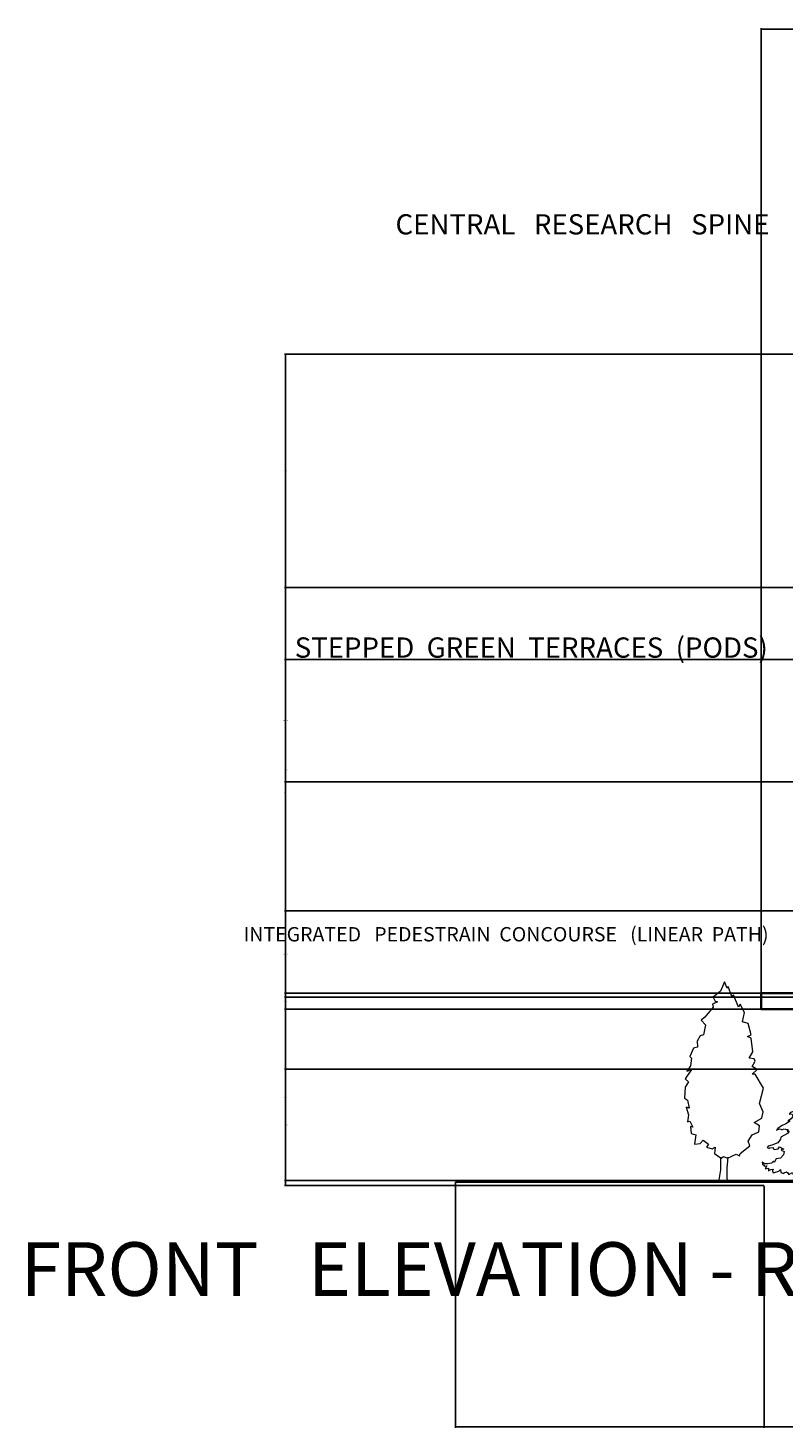
# Model space of a CAD drawing. Units: inches. Extents: x -160 to 434, y -145 to 103.
# Tile 1 of 7: x -160 to -26, y -145 to 103. Entities that reach past the tile are written whole.
import ezdxf

# ---------------------------------------------------------------- set-up
doc = ezdxf.new("R2010")
doc.units = ezdxf.units.IN
doc.header["$MEASUREMENT"] = 0
for name, color, linetype, lineweight in [('A-ANNO-DIMS', 2, 'Continuous', 18), ('A-ANNO-TEXT', 3, 'Continuous', 18), ('A-ELEV', 7, 'Continuous', 35), ('L-PLNT', 3, 'Continuous', 13)]:
    doc.layers.add(name, color=color, linetype=linetype, lineweight=lineweight)
doc.styles.get("Standard").update_dxf_attribs({"font": 'arial.ttf'})
doc.dimstyles.get("Standard").update_dxf_attribs({"dimtxt": 0.18, "dimasz": 0.18, "dimexe": 0.18, "dimexo": 0.0625, "dimgap": 0.09, "dimtad": 0, "dimtih": 1, "dimtoh": 1, "dimdec": 4, "dimzin": 0, "dimdsep": 46, "dimtxsty": 'Standard', "dimcen": 0.09, "dimadec": 0, "dimazin": 0, "dimtfac": 1, "dimtdec": 4, "dimtofl": 0, "dimtmove": 0, "dimatfit": 3, "dimfxl": 1, "dimtolj": 1, "dimtzin": 0, "dimarcsym": 0})

# ---------------------------------------------------------------- blocks, each defined once
blk = doc.blocks.new('*U2')
blk.add_lwpolyline([(-2.754, 191.699), (-6.78, 182.851), (-13.682, 176.953), (-11.956, 173.266), (-9.656, 172.529), (-14.257, 170.317), (-13.682, 167.368), (-21.733, 157.783), (-25.184, 154.834), (-21.158, 150.41), (-21.733, 147.461), (-22.884, 140.825), (-26.334, 140.087), (-29.21, 134.926), (-28.635, 129.028), (-32.661, 128.291), (-36.111, 120.18), (-34.386, 118.706), (-35.536, 111.333), (-38.987, 106.171), (-34.386, 107.646), (-40.712, 98.798), (-37.261, 95.849), (-40.712, 90.688), (-41.287, 80.366), (-38.412, 78.154), (-36.686, 70.781), (-39.562, 71.518), (-37.261, 64.145), (-38.412, 57.509), (-36.111, 58.247), (-33.236, 52.348), (-35.536, 53.086), (-34.961, 46.45), (-30.36, 44.975), (-31.51, 36.128), (-26.334, 36.865), (-23.459, 39.814), (-18.283, 36.128), (-20.008, 33.178), (-14.832, 31.704), (-11.956, 33.178), (-12.531, 27.28), (-6.205, 22.856), (-3.905, 24.331), (0.121, 22.856), (8.173, 26.543), (11.624, 25.068), (12.199, 27.28), (21.4, 34.653), (19.675, 39.077), (23.701, 44.975), (30.027, 47.924), (30.602, 53.823), (25.426, 56.772), (32.903, 61.196), (34.053, 67.094), (30.602, 75.205), (34.628, 89.951), (26.576, 103.222), (23.701, 103.222), (28.302, 107.646), (23.701, 110.595), (26.576, 115.756), (25.426, 117.968), (20.825, 118.706), (24.276, 124.604), (22.551, 137.876), (19.1, 139.35), (22.551, 140.825), (19.675, 151.884), (14.499, 153.359), (16.224, 162.207), (12.199, 170.317), (10.473, 167.368), (5.872, 179.165), (4.147, 177.69), (0.696, 187.275), (-0.454, 185.8)], close=True)
for points in [[(-6.813, 23.669), (-6.813, 11.669), (-8.627, 0)], [(0.387, 23.669), (-0.576, 13.271), (-0.576, 3.686), (0, 0)]]:
    blk.add_lwpolyline(points)
blk = doc.blocks.new('*U7')
for p, q in [((-9.75, 0), (-8.263, 7.598)), ((-8.263, 7.598), (-8.747, 14.105)), ((-0.771, 9.56), (-0.69, 11.833)), ((0, 0), (-0.771, 9.56))]:
    blk.add_line(p, q)
for points in [[(-3.9, 142.35), (-6.596, 132.037), (-10.801, 128.443), (-17.81, 126.047), (-20.614, 122.452), (-17.81, 123.65), (-15.007, 123.051), (-13.605, 118.858), (-16.876, 114.065), (-21.549, 111.07), (-22.951, 109.872), (-19.212, 110.471), (-19.68, 109.273), (-26.222, 105.079), (-34.633, 101.485), (-41.175, 96.693), (-43.511, 93.098), (-41.175, 94.296), (-36.969, 95.494), (-34.633, 94.296), (-32.764, 94.296), (-29.493, 95.494)], [(-3.759, 141.97), (-1.074, 131.643), (2.437, 127.141), (8.84, 124.493), (6.568, 124.493), (4.09, 123.169), (4.296, 121.846), (7.807, 117.874), (16.069, 116.02), (10.492, 115.226), (5.535, 113.372), (6.981, 112.843), (5.948, 110.989), (10.286, 112.048), (6.775, 109.401), (11.732, 108.077), (9.873, 107.282), (13.797, 102.516), (21.852, 101.192), (25.983, 103.84), (28.048, 106.488), (27.842, 105.164), (27.429, 101.457), (24.124, 97.75), (23.091, 93.513), (19.58, 93.513), (23.505, 91.66), (28.255, 90.866), (31.973, 91.925), (29.081, 89.806), (24.537, 88.747), (26.809, 88.218), (22.472, 86.099), (24.95, 85.57), (17.308, 84.246), (21.852, 80.804), (29.081, 79.215), (36.723, 80.009), (39.821, 82.392), (40.028, 80.009), (45.398, 76.567)], [(-29.25, 95.55), (-25.287, 94.296), (-22.016, 94.296), (-23.885, 91.301), (-20.614, 91.301), (-23.418, 87.108), (-35.567, 80.518), (-36.035, 76.924), (-41.175, 70.334), (-52.389, 65.542), (-58.931, 63.744), (-60.8, 61.348), (-57.062, 59.551), (-56.128, 60.749), (-50.987, 61.348), (-48.184, 57.754), (-40.707, 58.952), (-38.371, 62.546), (-30.427, 58.353), (-33.698, 58.353), (-35.1, 56.556), (-29.493, 54.159), (-30.894, 48.169), (-36.035, 41.579), (-44.446, 40.381), (-48.184, 33.791), (-49.118, 36.188), (-52.857, 32.593), (-59.399, 31.395), (-65.473, 31.395), (-70.146, 34.39), (-69.679, 30.796), (-66.875, 28.999), (-65.941, 27.202), (-61.268, 27.801), (-64.539, 22.409), (-58.464, 23.607), (-58.464, 18.815), (-54.258, 21.211), (-49.586, 21.81), (-50.987, 18.815), (-50.52, 15.82), (-47.249, 15.82), (-39.306, 18.216), (-36.502, 21.211), (-35.567, 15.82), (-30.427, 13.423), (-29.493, 15.221), (-25.287, 17.018), (-22.951, 15.221), (-21.081, 11.626), (-14.539, 15.82), (-13.138, 11.626), (-6.128, 15.82), (-4.726, 12.824), (10.226, 9.23), (5.554, 12.225), (13.497, 10.428), (10.226, 12.824), (16.768, 13.423), (22.376, 11.626), (27.516, 12.225), (21.909, 15.221), (34.993, 15.221), (44.806, 12.824), (41.535, 16.419), (42.469, 19.414), (49.011, 14.023), (56.487, 13.423), (66.768, 17.018), (64.431, 18.815), (60.226, 18.216), (60.226, 20.612), (56.955, 20.612), (56.955, 24.206), (54.151, 24.206), (51.348, 28.4), (50.413, 26.004), (47.609, 26.603), (43.871, 30.197), (38.731, 30.197), (34.525, 30.197), (27.983, 33.791), (38.731, 40.98), (47.609, 40.98), (45.273, 45.773), (52.282, 48.169), (56.955, 47.57), (55.086, 52.362), (48.544, 51.164), (39.198, 52.362), (35.927, 56.556), (33.123, 55.357), (31.254, 59.551), (27.049, 58.353), (22.376, 62.546), (28.451, 65.542), (39.198, 66.74), (41.535, 72.131), (45.273, 76.325)]]:
    blk.add_lwpolyline(points)
blk = doc.blocks.new('*D12')
at = {"layer": 'A-ANNO-DIMS', "color": 0, "lineweight": -2, "transparency": 16777216}
for p, q in [((-84.07, -101.41), (-84.07, -144.81)), ((403.75, -101.41), (403.75, -144.81)), ((-83.89, -144.63), (159.44, -144.63)), ((403.57, -144.63), (160.24, -144.63))]:
    blk.add_line(p, q, dxfattribs=at)
at = {"layer": 'A-ANNO-DIMS', "color": 0, "transparency": 16777216}
for points in [[(-83.89, -144.6), (-83.89, -144.66), (-84.07, -144.63)], [(403.57, -144.6), (403.57, -144.66), (403.75, -144.63)]]:
    blk.add_solid(points, dxfattribs=at)
at = {"layer": 'Defpoints', "color": 0, "transparency": 16777216}
for p in [(-84.07, -101.35), (403.75, -101.35), (403.75, -144.63)]:
    blk.add_point(p, dxfattribs=at)
at = {"layer": 'A-ANNO-DIMS', "color": 0, "transparency": 16777216, "insert": (159.84, -144.63), "char_height": 0.18, "attachment_point": 5}
blk.add_mtext('\\A1;487.8', dxfattribs=at)
blk = doc.blocks.new('*D13')
at = {"layer": 'A-ANNO-DIMS', "color": 0, "lineweight": -2, "transparency": 16777216}
for p, q in [((-30.14, -70.84), (-114.3, -70.84)), ((-114.12, -71.02), (-114.12, -86.22)), ((-114.12, -101.79), (-114.12, -86.59)), ((-29.6, -101.97), (-114.3, -101.97))]:
    blk.add_line(p, q, dxfattribs=at)
at = {"layer": 'A-ANNO-DIMS', "color": 0, "transparency": 16777216}
for points in [[(-114.15, -71.02), (-114.09, -71.02), (-114.12, -70.84)], [(-114.15, -101.79), (-114.09, -101.79), (-114.12, -101.97)]]:
    blk.add_solid(points, dxfattribs=at)
at = {"layer": 'Defpoints', "color": 0, "transparency": 16777216}
for p in [(-114.12, -70.84), (-30.07, -70.84), (-29.54, -101.97)]:
    blk.add_point(p, dxfattribs=at)
at = {"layer": 'A-ANNO-DIMS', "color": 0, "transparency": 16777216, "insert": (-114.12, -86.41), "char_height": 0.18, "attachment_point": 5}
blk.add_mtext('\\A1;31.14', dxfattribs=at)
blk = doc.blocks.new('*D14')
at = {"layer": 'A-ANNO-DIMS', "color": 0, "lineweight": -2, "transparency": 16777216}
for p, q in [((-30.14, -67.97), (-114.3, -67.97)), ((-114.12, -68.15), (-114.12, -69.22)), ((-30.14, -70.84), (-114.3, -70.84)), ((-114.12, -70.66), (-114.12, -69.59))]:
    blk.add_line(p, q, dxfattribs=at)
at = {"layer": 'A-ANNO-DIMS', "color": 0, "transparency": 16777216}
for points in [[(-114.15, -68.15), (-114.09, -68.15), (-114.12, -67.97)], [(-114.15, -70.66), (-114.09, -70.66), (-114.12, -70.84)]]:
    blk.add_solid(points, dxfattribs=at)
at = {"layer": 'Defpoints', "color": 0, "transparency": 16777216}
for p in [(-114.12, -67.97), (-30.07, -67.97), (-30.07, -70.84)]:
    blk.add_point(p, dxfattribs=at)
at = {"layer": 'A-ANNO-DIMS', "color": 0, "transparency": 16777216, "insert": (-114.12, -69.41), "char_height": 0.18, "attachment_point": 5}
blk.add_mtext('\\A1;2.863', dxfattribs=at)
blk = doc.blocks.new('*D15')
at = {"layer": 'A-ANNO-DIMS', "color": 0, "lineweight": -2, "transparency": 16777216}
for p, q in [((2.83, 44.89), (-114.3, 44.89)), ((-114.12, 44.71), (-114.12, -28.36)), ((-114.12, -101.79), (-114.12, -28.72)), ((-29.6, -101.97), (-114.3, -101.97))]:
    blk.add_line(p, q, dxfattribs=at)
at = {"layer": 'A-ANNO-DIMS', "color": 0, "transparency": 16777216}
for points in [[(-114.15, 44.71), (-114.09, 44.71), (-114.12, 44.89)], [(-114.15, -101.79), (-114.09, -101.79), (-114.12, -101.97)]]:
    blk.add_solid(points, dxfattribs=at)
at = {"layer": 'Defpoints', "color": 0, "transparency": 16777216}
for p in [(-114.12, 44.89), (2.89, 44.89), (-29.54, -101.97)]:
    blk.add_point(p, dxfattribs=at)
at = {"layer": 'A-ANNO-DIMS', "color": 0, "transparency": 16777216, "insert": (-114.12, -28.54), "char_height": 0.18, "attachment_point": 5}
blk.add_mtext('\\A1;146.87', dxfattribs=at)
blk = doc.blocks.new('*D16')
at = {"layer": 'A-ANNO-DIMS', "color": 0, "lineweight": -2, "transparency": 16777216}
for p, q in [((-29.54, -102.04), (-29.54, -144.81)), ((2.66, -101.41), (2.66, -144.81)), ((-29.36, -144.63), (-13.76, -144.63)), ((2.48, -144.63), (-13.12, -144.63))]:
    blk.add_line(p, q, dxfattribs=at)
at = {"layer": 'A-ANNO-DIMS', "color": 0, "transparency": 16777216}
for points in [[(-29.36, -144.6), (-29.36, -144.66), (-29.54, -144.63)], [(2.48, -144.6), (2.48, -144.66), (2.66, -144.63)]]:
    blk.add_solid(points, dxfattribs=at)
at = {"layer": 'Defpoints', "color": 0, "transparency": 16777216}
for p in [(2.66, -101.35), (-29.54, -101.97), (2.66, -144.63)]:
    blk.add_point(p, dxfattribs=at)
at = {"layer": 'A-ANNO-DIMS', "color": 0, "transparency": 16777216, "insert": (-13.44, -144.63), "char_height": 0.18, "attachment_point": 5}
blk.add_mtext('\\A1;32.2', dxfattribs=at)
blk = doc.blocks.new('*D25')
at = {"layer": 'A-ANNO-DIMS', "color": 0, "lineweight": -2, "transparency": 16777216}
for p, q in [((78.9, -81.45), (-114.3, -81.45)), ((-114.12, -81.63), (-114.12, -91.1)), ((-114.12, -100.92), (-114.12, -91.46)), ((79.28, -101.1), (-114.3, -101.1))]:
    blk.add_line(p, q, dxfattribs=at)
at = {"layer": 'A-ANNO-DIMS', "color": 0, "transparency": 16777216}
for points in [[(-114.15, -81.63), (-114.09, -81.63), (-114.12, -81.45)], [(-114.15, -100.92), (-114.09, -100.92), (-114.12, -101.1)]]:
    blk.add_solid(points, dxfattribs=at)
at = {"layer": 'Defpoints', "color": 0, "transparency": 16777216}
for p in [(78.96, -81.45), (-114.12, -101.1), (79.34, -101.1)]:
    blk.add_point(p, dxfattribs=at)
at = {"layer": 'A-ANNO-DIMS', "color": 0, "transparency": 16777216, "insert": (-114.12, -91.28), "char_height": 0.18, "attachment_point": 5}
blk.add_mtext('\\A1;19.646', dxfattribs=at)
blk = doc.blocks.new('*D29')
at = {"layer": 'A-ANNO-DIMS', "color": 0, "lineweight": -2, "transparency": 16777216}
for p, q in [((2.83, 44.89), (-114.3, 44.89)), ((-114.12, 44.71), (-114.12, 24.46)), ((-114.12, 3.84), (-114.12, 24.1)), ((2.83, 3.66), (-114.3, 3.66))]:
    blk.add_line(p, q, dxfattribs=at)
at = {"layer": 'A-ANNO-DIMS', "color": 0, "transparency": 16777216}
for points in [[(-114.15, 44.71), (-114.09, 44.71), (-114.12, 44.89)], [(-114.15, 3.84), (-114.09, 3.84), (-114.12, 3.66)]]:
    blk.add_solid(points, dxfattribs=at)
at = {"layer": 'Defpoints', "color": 0, "transparency": 16777216}
for p in [(2.89, 44.89), (-114.12, 3.66), (2.89, 3.66)]:
    blk.add_point(p, dxfattribs=at)
at = {"layer": 'A-ANNO-DIMS', "color": 0, "transparency": 16777216, "insert": (-114.12, 24.28), "char_height": 0.18, "attachment_point": 5}
blk.add_mtext('\\A1;41.23', dxfattribs=at)
blk = doc.blocks.new('*D30')
at = {"layer": 'A-ANNO-DIMS', "color": 0, "lineweight": -2, "transparency": 16777216}
for p, q in [((2.83, 3.66), (-114.3, 3.66)), ((-114.12, 3.48), (-114.12, -32.35)), ((-114.12, -68.55), (-114.12, -32.72)), ((-9.37, -68.73), (-114.3, -68.73))]:
    blk.add_line(p, q, dxfattribs=at)
at = {"layer": 'A-ANNO-DIMS', "color": 0, "transparency": 16777216}
for points in [[(-114.15, 3.48), (-114.09, 3.48), (-114.12, 3.66)], [(-114.15, -68.55), (-114.09, -68.55), (-114.12, -68.73)]]:
    blk.add_solid(points, dxfattribs=at)
at = {"layer": 'Defpoints', "color": 0, "transparency": 16777216}
for p in [(-114.12, 3.66), (2.89, 3.66), (-9.31, -68.73)]:
    blk.add_point(p, dxfattribs=at)
at = {"layer": 'A-ANNO-DIMS', "color": 0, "transparency": 16777216, "insert": (-114.12, -32.54), "char_height": 0.18, "attachment_point": 5}
blk.add_mtext('\\A1;72.4', dxfattribs=at)
blk = doc.blocks.new('*D34')
at = {"layer": 'A-ANNO-DIMS', "color": 0, "lineweight": -2, "transparency": 16777216}
for p, q in [((67.03, -9.07), (-114.3, -9.07)), ((-114.12, -9.25), (-114.12, -19.67)), ((-114.12, -30.46), (-114.12, -20.04)), ((66.72, -30.64), (-114.3, -30.64))]:
    blk.add_line(p, q, dxfattribs=at)
at = {"layer": 'A-ANNO-DIMS', "color": 0, "transparency": 16777216}
for points in [[(-114.15, -9.25), (-114.09, -9.25), (-114.12, -9.07)], [(-114.15, -30.46), (-114.09, -30.46), (-114.12, -30.64)]]:
    blk.add_solid(points, dxfattribs=at)
at = {"layer": 'Defpoints', "color": 0, "transparency": 16777216}
for p in [(67.09, -9.07), (-114.12, -30.64), (66.78, -30.64)]:
    blk.add_point(p, dxfattribs=at)
at = {"layer": 'A-ANNO-DIMS', "color": 0, "transparency": 16777216, "insert": (-114.12, -19.85), "char_height": 0.18, "attachment_point": 5}
blk.add_mtext('\\A1;21.567', dxfattribs=at)
blk = doc.blocks.new('*D36')
at = {"layer": 'A-ANNO-DIMS', "color": 0, "lineweight": -2, "transparency": 16777216}
for p, q in [((-9.51, -53.43), (-114.3, -53.43)), ((-114.12, -53.61), (-114.12, -60.9)), ((-114.12, -68.55), (-114.12, -61.26)), ((-9.37, -68.73), (-114.3, -68.73))]:
    blk.add_line(p, q, dxfattribs=at)
at = {"layer": 'A-ANNO-DIMS', "color": 0, "transparency": 16777216}
for points in [[(-114.15, -53.61), (-114.09, -53.61), (-114.12, -53.43)], [(-114.15, -68.55), (-114.09, -68.55), (-114.12, -68.73)]]:
    blk.add_solid(points, dxfattribs=at)
at = {"layer": 'Defpoints', "color": 0, "transparency": 16777216}
for p in [(-9.45, -53.43), (-114.12, -68.73), (-9.31, -68.73)]:
    blk.add_point(p, dxfattribs=at)
at = {"layer": 'A-ANNO-DIMS', "color": 0, "transparency": 16777216, "insert": (-114.12, -61.08), "char_height": 0.18, "attachment_point": 5}
blk.add_mtext('\\A1;15.304', dxfattribs=at)
blk = doc.blocks.new('*D47')
at = {"layer": 'A-ANNO-DIMS', "color": 0, "lineweight": -2, "transparency": 16777216}
for p, q in [((-30.07, -67.91), (-30.07, 102.5)), ((-29.89, 102.32), (-20.23, 102.32)), ((-9.63, 102.32), (-19.3, 102.32)), ((-9.45, -53.37), (-9.45, 102.5))]:
    blk.add_line(p, q, dxfattribs=at)
at = {"layer": 'A-ANNO-DIMS', "color": 0, "transparency": 16777216}
for points in [[(-29.89, 102.35), (-29.89, 102.29), (-30.07, 102.32)], [(-9.63, 102.35), (-9.63, 102.29), (-9.45, 102.32)]]:
    blk.add_solid(points, dxfattribs=at)
at = {"layer": 'Defpoints', "color": 0, "transparency": 16777216}
for p in [(-9.45, 102.32), (-9.45, -53.43), (-30.07, -67.97)]:
    blk.add_point(p, dxfattribs=at)
at = {"layer": 'A-ANNO-DIMS', "color": 0, "transparency": 16777216, "insert": (-19.76, 102.32), "char_height": 0.18, "attachment_point": 5}
blk.add_mtext('\\A1;20.625', dxfattribs=at)

msp = doc.modelspace()

# ---------------------------------------------------------------- linework, layer by layer
at = {"layer": 'A-ELEV'}
for p, q in [((-12.2824, -67.9742), (-30.0745, -67.9742)), ((-30.0745, -67.9742), (-30.0745, -70.8373)), ((-30.0745, -70.8373), (-12.2824, -70.8373)), ((2.6577, -101.346), (-84.0722, -101.346))]:
    msp.add_line(p, q, dxfattribs=at)

# ---------------------------------------------------------------- block references
at = {"layer": 'L-PLNT'}
for name, p, xscale, yscale, zscale in [('*U2', (-36.0092, -101.3328), 0.1843091790693797, 0.1843091790693797, 0.1843091790693797), ('*U7', (-23.1588, -101.1712), 0.0961203238098615, 0.0961203238098615, 0.0961203238098615)]:
    msp.add_blockref(name, p, dxfattribs=dict(at, xscale=xscale, yscale=yscale, zscale=zscale))

# ---------------------------------------------------------------- texts
at = {"layer": 'A-ANNO-TEXT'}
for s, height, p in [('CENTRAL   RESEARCH   SPINE', 3.579169, (-94.6752, 66.0288)), ('STEPPED  GREEN  TERRACES  (PODS)', 3.579169, (-112.4851, -8.7354)), ('INTEGRATED   PEDESTRAIN  CONCOURSE   (LINEAR  PATH)', 2.531175, (-121.5214, -58.8538)), ('FRONT   ELEVATION - RESEARCH   SPINE   AND  COLLABORATION   PODS  (NEW   CONCEPT)', 9.480943, (-160.9184, -121.4719))]:
    msp.add_text(s, height=height, dxfattribs=at).set_placement(p)

# ---------------------------------------------------------------- dimensions: what is measured, and where the dimension line sits
at = {"layer": 'A-ANNO-DIMS'}
for base, p1, p2, override, picture, middle in [((-9.4492, 102.3218), (-30.0745, -67.9742), (-9.4492, -53.4308), {"dimdec": 3, "dimlfac": 1, "dimrnd": 0, "dimzin": 0, "dimdsep": 46, "dimlunit": 2}, '*D47', (-19.7619, 102.3218)), ((403.7477, -144.6322), (-84.0722, -101.346), (403.7477, -101.346), {"dimdec": 1, "dimlfac": 1, "dimrnd": 0, "dimzin": 0, "dimdsep": 46, "dimlunit": 2}, '*D12', (159.8378, -144.6322)), ((2.6577, -144.6322), (-29.5407, -101.9747), (2.6577, -101.346), {"dimdec": 1, "dimlfac": 1, "dimrnd": 0, "dimzin": 0, "dimdsep": 46, "dimlunit": 2}, '*D16', (-13.4415, -144.6322))]:
    dim = msp.add_linear_dim(base=base, p1=p1, p2=p2, dimstyle='Standard', override=override, dxfattribs=at)
    dim.commit()
    dim.dimension.update_dxf_attribs({"geometry": picture, "text_midpoint": middle})
for base, p1, p2, override, picture, middle in [((-114.1222, 44.8926), (-29.5407, -101.9747), (2.8933, 44.8926), {"dimdec": 2, "dimlfac": 1, "dimrnd": 0, "dimzin": 0, "dimdsep": 46, "dimlunit": 2}, '*D15', (-114.1222, -28.5411)), ((-114.1222, 3.6646), (2.8933, 44.8926), (2.8933, 3.6646), {"dimdec": 2, "dimlfac": 1, "dimrnd": 0, "dimzin": 0, "dimdsep": 46, "dimlunit": 2}, '*D29', (-114.1222, 24.2786)), ((-114.1222, 3.6646), (-9.3089, -68.735), (2.8933, 3.6646), {"dimdec": 1, "dimlfac": 1, "dimrnd": 0, "dimzin": 0, "dimdsep": 46, "dimlunit": 2}, '*D30', (-114.1222, -32.5352)), ((-114.12224, -30.63792), (67.09448, -9.07136), (66.78146, -30.63791), {"dimdec": 3, "dimlfac": 1, "dimrnd": 0, "dimzin": 0, "dimdsep": 46, "dimlunit": 2}, '*D34', (-114.12224, -19.85463)), ((-114.1222, -68.735), (-9.4492, -53.4308), (-9.3089, -68.735), {"dimdec": 3, "dimlfac": 1, "dimrnd": 0, "dimzin": 0, "dimdsep": 46, "dimlunit": 2}, '*D36', (-114.1222, -61.0829)), ((-114.1222, -67.9742), (-30.0745, -70.8373), (-30.0745, -67.9742), {"dimdec": 3, "dimlfac": 1, "dimrnd": 0, "dimzin": 0, "dimdsep": 46, "dimlunit": 2}, '*D14', (-114.1222, -69.4057)), ((-114.1222, -70.8373), (-29.5407, -101.9747), (-30.0745, -70.8373), {"dimdec": 2, "dimlfac": 1, "dimrnd": 0, "dimzin": 0, "dimdsep": 46, "dimlunit": 2}, '*D13', (-114.1222, -86.406)), ((-114.1222, -101.1003), (78.9633, -81.4546), (79.3401, -101.1003), {"dimdec": 3, "dimlfac": 1, "dimrnd": 0, "dimzin": 0, "dimdsep": 46, "dimlunit": 2}, '*D25', (-114.1222, -91.2774))]:
    dim = msp.add_linear_dim(base=base, p1=p1, p2=p2, angle=90, dimstyle='Standard', override=override, dxfattribs=at)
    dim.commit()
    dim.dimension.update_dxf_attribs({"geometry": picture, "text_midpoint": middle})

doc.saveas('drawing.dxf')
